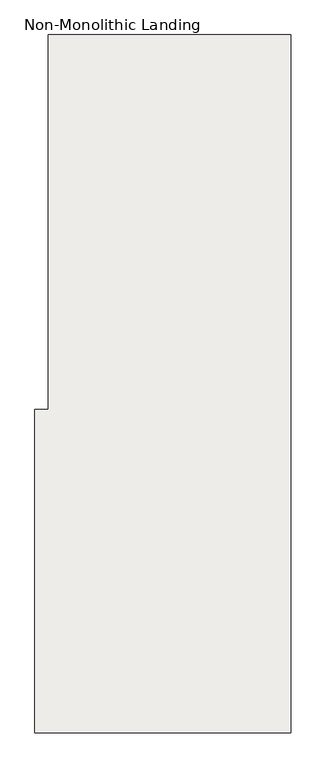
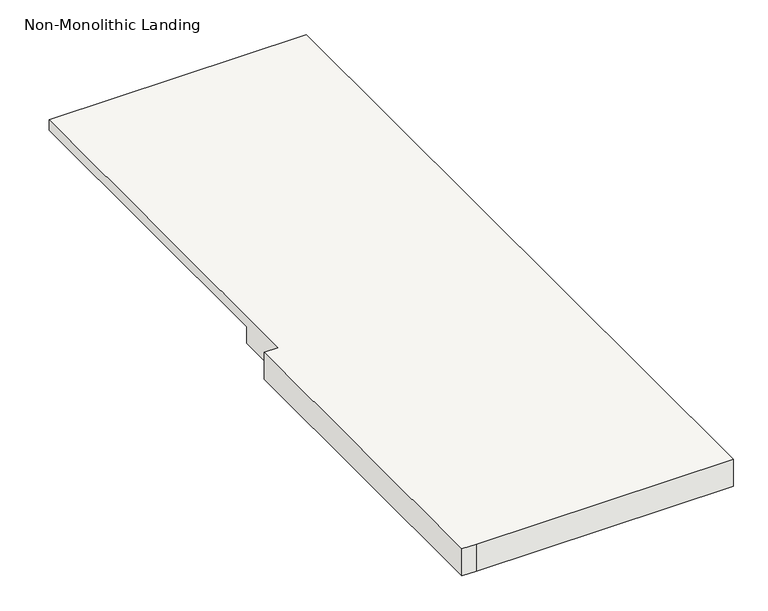
"""IFC4 building model written with IfcOpenShell, lengths in millimetres: slab geometry, Non-Monolithic Landing."""

from ifc_helpers import new_model, si_unit, origin, place, context, project, spatial, faceted_brep, source, transform, mapped, element, save


def non_monolithic_landing_1e13c623(model_context):
    return source(origin(), model_context, "Body", "Brep", [
        faceted_brep([(-3732.7409298, -3238.4779636, 7981.95), (-3707.3409298, -3238.4779636, 7956.55), (-3707.3409298, -3848.0779636, 7956.55), (-3732.7409298, -3848.0779636, 7981.95), (-3732.7409298, -3945.3664375, 8001.0), (-3758.1409298, -3945.3664375, 8001.0), (-3758.1409298, -4554.9664375, 8001.0), (-3732.7409298, -4554.9664375, 8001.0), (-3275.5409298, -4554.9664375, 8001.0), (-3275.5409298, -3238.4779636, 8001.0), (-3732.7409298, -3238.4779636, 8001.0), (-3707.3409298, -3848.0779636, 7950.2), (-3707.3409298, -3238.4779636, 7950.2), (-3275.5409298, -3238.4779636, 7950.2), (-3275.5409298, -4554.9664375, 7950.2), (-3732.7409298, -4554.9664375, 7950.2), (-3758.1409298, -4554.9664375, 7950.2), (-3758.1409298, -3945.3664375, 7950.2), (-3732.7409298, -3945.3664375, 7950.2), (-3732.7409298, -3848.0779636, 7950.2)], [[[0, 1, 2, 3]], [[4, 5, 6, 7, 8, 9, 10]], [[11, 12, 13, 14, 15, 16, 17, 18, 19]], [[12, 11, 2, 1]], [[11, 19, 3, 2]], [[4, 10, 0, 3, 19, 18]], [[5, 4, 18, 17]], [[6, 5, 17, 16]], [[7, 6, 16, 15]], [[8, 7, 15, 14]], [[9, 8, 14, 13]], [[10, 9, 13, 12, 1, 0]]]),
    ])


if __name__ == "__main__":
    model = new_model("IFC4")
    model_context = context("Model", 3, world=origin())
    ifc_project = project(units=[si_unit("LENGTHUNIT", "METRE", prefix="MILLI")], contexts=[model_context])
    site = spatial("IfcSite", under=ifc_project)
    building = spatial("IfcBuilding", under=site)
    placement = place(None, origin())
    non_monolithic_landing_shape = non_monolithic_landing_1e13c623(model_context)
    element("IfcSlab", 1, ObjectType="Non-Monolithic Landing", at=placement, inside=building, context=model_context, shape_type="MappedRepresentation", body=[
        mapped(non_monolithic_landing_shape, transform((0.0, 0.0, 0.0), x_axis=(1.0, 0.0, 0.0), y_axis=(0.0, 1.0, 0.0), z_axis=(0.0, 0.0, 1.0))),
    ])
    save(model, "model.ifc")
